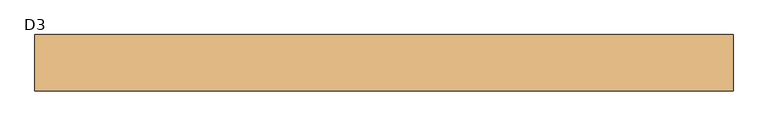
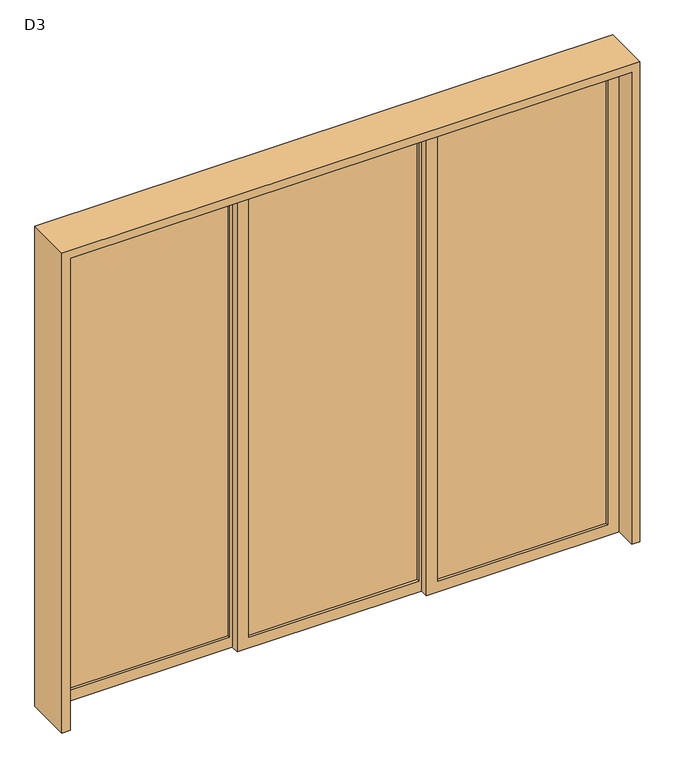
"""IFC4 building model written with IfcOpenShell, lengths in millimetres: door geometry, D3."""

from ifc_helpers import new_model, si_unit, frame, origin, place, context, project, spatial, polyline, outline, extrude, source, transform, mapped, element, save


def d3_8cc66dcc(model_context):
    return source(origin(), model_context, "Body", "SweptSolid", [
        extrude(outline(polyline([(1380.7580012, 5.8333333), (563.2580012, 5.8333333), (563.2580012, 19.1666667), (1380.7580012, 19.1666667), (1380.7580012, 5.8333333)])), frame((0.0, 0.0, 55.0), z_axis=(0.0, 0.0, 1.0), x_axis=(1.0, 0.0, 0.0)), (0.0, 0.0, 1.0), 2290.0),
        extrude(outline(polyline([(0.0, 1435.7580012), (2400.0, 1435.7580012), (2400.0, 508.2580012), (0.0, 508.2580012), (0.0, 1435.7580012)]), holes=[polyline([(55.0, 1380.7580012), (55.0, 563.2580012), (2345.0, 563.2580012), (2345.0, 1380.7580012), (55.0, 1380.7580012)])]), frame((0.0, -7.5, 0.0), z_axis=(0.0, 1.0, 0.0), x_axis=(0.0, 0.0, 1.0)), (0.0, 0.0, 1.0), 40.0),
        extrude(outline(polyline([(494.9246679, 45.8333333), (-322.5753321, 45.8333333), (-322.5753321, 59.1666667), (494.9246679, 59.1666667), (494.9246679, 45.8333333)])), frame((0.0, 0.0, 55.0), z_axis=(0.0, 0.0, 1.0), x_axis=(1.0, 0.0, 0.0)), (0.0, 0.0, 1.0), 2290.0),
        extrude(outline(polyline([(0.0, 549.9246679), (2400.0, 549.9246679), (2400.0, -377.5753321), (0.0, -377.5753321), (0.0, 549.9246679)]), holes=[polyline([(55.0, 494.9246679), (55.0, -322.5753321), (2345.0, -322.5753321), (2345.0, 494.9246679), (55.0, 494.9246679)])]), frame((0.0, 32.5, 0.0), z_axis=(0.0, 1.0, 0.0), x_axis=(0.0, 0.0, 1.0)), (0.0, 0.0, 1.0), 40.0),
        extrude(outline(polyline([(-391.7419988, 85.8333333), (-1209.2419988, 85.8333333), (-1209.2419988, 99.1666667), (-391.7419988, 99.1666667), (-391.7419988, 85.8333333)])), frame((0.0, 0.0, 55.0), z_axis=(0.0, 0.0, 1.0), x_axis=(1.0, 0.0, 0.0)), (0.0, 0.0, 1.0), 2290.0),
        extrude(outline(polyline([(0.0, -336.7419988), (2400.0, -336.7419988), (2400.0, -1264.2419988), (0.0, -1264.2419988), (0.0, -336.7419988)]), holes=[polyline([(55.0, -391.7419988), (55.0, -1209.2419988), (2345.0, -1209.2419988), (2345.0, -391.7419988), (55.0, -391.7419988)])]), frame((0.0, 72.5, 0.0), z_axis=(0.0, 1.0, 0.0), x_axis=(0.0, 0.0, 1.0)), (0.0, 0.0, 1.0), 40.0),
        extrude(outline(polyline([(0.0, -1264.2419988), (2400.0, -1264.2419988), (2400.0, 1435.7580012), (0.0, 1435.7580012), (0.0, 1475.7580012), (2440.0, 1475.7580012), (2440.0, -1304.2419988), (0.0, -1304.2419988), (0.0, -1264.2419988)])), frame((0.0, -112.5, 0.0), z_axis=(0.0, 1.0, 0.0), x_axis=(0.0, 0.0, 1.0)), (0.0, 0.0, 1.0), 225.0),
    ])


if __name__ == "__main__":
    model = new_model("IFC4")
    model_context = context("Model", 3, world=origin())
    ifc_project = project(units=[si_unit("LENGTHUNIT", "METRE", prefix="MILLI")], contexts=[model_context])
    site = spatial("IfcSite", under=ifc_project)
    building = spatial("IfcBuilding", under=site)
    placement = place(None, origin())
    d3_shape = d3_8cc66dcc(model_context)
    element("IfcDoor", 1, ObjectType="D3", at=placement, inside=building, context=model_context, shape_type="MappedRepresentation", body=[
        mapped(d3_shape, transform((0.0, 0.0, 0.0), x_axis=(1.0, 0.0, 0.0), y_axis=(0.0, 1.0, 0.0), z_axis=(0.0, 0.0, 1.0))),
    ])
    save(model, "model.ifc")

# Revit data of these elements
# Type "D3"
#   Type Mark = "52"
#   Operation = "UserDefined"
#   Width = 2700 mm
#   Thickness = 40 mm
#   Rough Width = 2780 mm
#   Rough Height = 2440 mm
#   Panel Width = 927.5 mm
#   Panel Frame = 55 mm
#   Height = 2400 mm
#   Frame Depth = 40 mm
#   Glass Material = Sliding Door Glass
#   Frame Material = Sliding Door Frame
#   Function = (empty or 0)
# Element 1 (IfcDoor, "D3")
#   Materials on its faces: "Sliding Door Frame", "Sliding Door Glass"
# Materials
#   "Sliding Door Glass": colour RGB 247 247 247, transparency 0.68
#   "Sliding Door Frame": colour RGB 160 107 8, transparency 0
